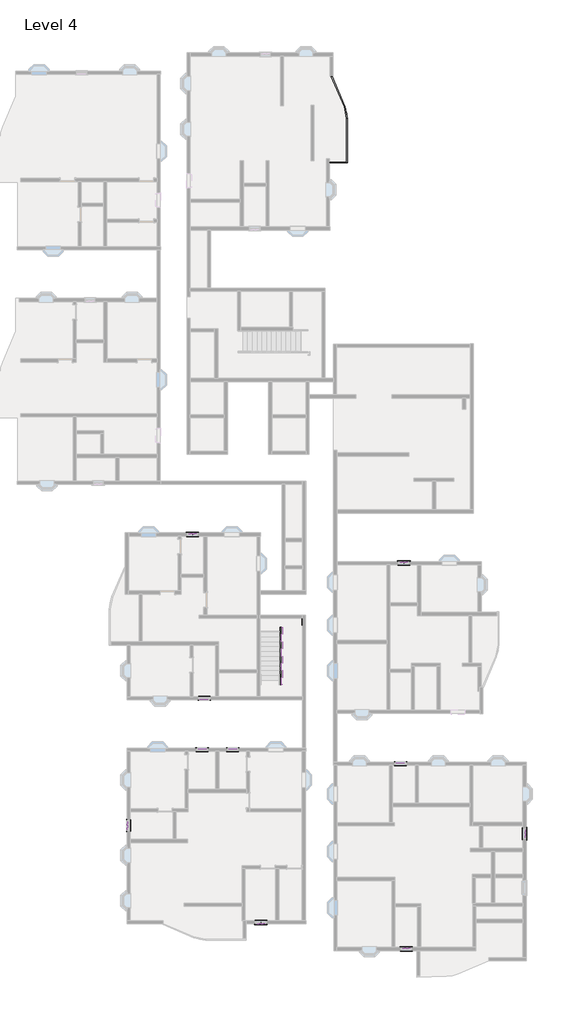
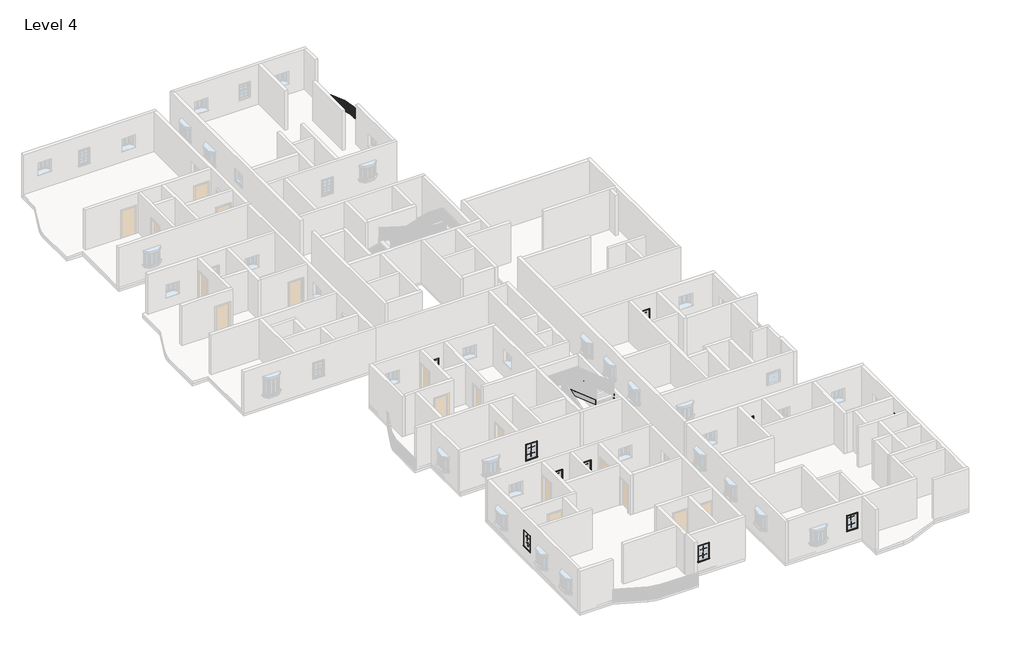
# One storey, part 13 of 14: 40 proxies, 6 members, 1 railing.
"""IFC4 building model written with IfcOpenShell, lengths in millimetres."""

from ifc_helpers import new_model, si_unit, frame, origin, place, context, project, spatial, polyline, circle_curve, outline, extrude, transform, mapped, element, save
from ifc_brep_helpers import plane_surface, cylinder_surface, revolved_surface, advanced_brep
from components import muntin_pattern_2x2_muntin_pattern_2x2_c35c595f, trim_window_exterior_flat_with_sill_e38017c9, trim_window_interior_flat_picture_frame_d728ed12

model = new_model("IFC4")

# Units and contexts
model_context = context("Model", 3, world=origin())
ifc_project = project(units=[si_unit("LENGTHUNIT", "METRE", prefix="MILLI")], contexts=[model_context])

# Site, building, storey
site = spatial("IfcSite", under=ifc_project)
building = spatial("IfcBuilding", under=site)
storey = spatial("IfcBuildingStorey", under=building, Name="Level 4", Elevation=9144.0)

# Proxies
placement = place(None, origin())
muntin_pattern_2x2_muntin_pattern_2x2_shape = muntin_pattern_2x2_muntin_pattern_2x2_c35c595f(model_context)
element("IfcBuildingElementProxy", 1, Name="Muntin Pattern_2x2 : Muntin Pattern_2x2", ObjectType="Muntin Pattern_2x2 : Muntin Pattern_2x2", at=placement, inside=storey, context=model_context, shape_type="MappedRepresentation", body=[
    mapped(muntin_pattern_2x2_muntin_pattern_2x2_shape, transform((-8150.287215, -357.5666506, 10614.025), x_axis=(1.0, 0.0, 0.0), y_axis=(0.0, 1.0, 0.0), z_axis=(0.0, 0.0, 1.0))),
])
element("IfcBuildingElementProxy", 2, Name="Muntin Pattern_2x2 : Muntin Pattern_2x2", ObjectType="Muntin Pattern_2x2 : Muntin Pattern_2x2", at=placement, inside=storey, context=model_context, shape_type="MappedRepresentation", body=[
    mapped(muntin_pattern_2x2_muntin_pattern_2x2_shape, transform((-8150.287215, -402.0166506, 10134.6), x_axis=(1.0, 0.0, 0.0), y_axis=(0.0, 1.0, 0.0), z_axis=(0.0, 0.0, 1.0))),
])
element("IfcBuildingElementProxy", 3, Name="Muntin Pattern_2x2 : Muntin Pattern_2x2", ObjectType="Muntin Pattern_2x2 : Muntin Pattern_2x2", at=placement, inside=storey, context=model_context, shape_type="MappedRepresentation", body=[
    mapped(muntin_pattern_2x2_muntin_pattern_2x2_shape, transform((-7397.812215, -10854.1166506, 10614.025), x_axis=(-1.0, 0.0, 0.0), y_axis=(0.0, -1.0, 0.0), z_axis=(0.0, 0.0, 1.0))),
])
element("IfcBuildingElementProxy", 4, Name="Muntin Pattern_2x2 : Muntin Pattern_2x2", ObjectType="Muntin Pattern_2x2 : Muntin Pattern_2x2", at=placement, inside=storey, context=model_context, shape_type="MappedRepresentation", body=[
    mapped(muntin_pattern_2x2_muntin_pattern_2x2_shape, transform((-7397.812215, -10809.6666506, 10134.6), x_axis=(-1.0, 0.0, 0.0), y_axis=(0.0, -1.0, 0.0), z_axis=(0.0, 0.0, 1.0))),
])
element("IfcBuildingElementProxy", 5, Name="Muntin Pattern_2x2 : Muntin Pattern_2x2", ObjectType="Muntin Pattern_2x2 : Muntin Pattern_2x2", at=placement, inside=storey, context=model_context, shape_type="MappedRepresentation", body=[
    mapped(muntin_pattern_2x2_muntin_pattern_2x2_shape, transform((-7540.687215, -13997.3666506, 10614.025), x_axis=(1.0, 0.0, 0.0), y_axis=(0.0, 1.0, 0.0), z_axis=(0.0, 0.0, 1.0))),
])
element("IfcBuildingElementProxy", 6, Name="Muntin Pattern_2x2 : Muntin Pattern_2x2", ObjectType="Muntin Pattern_2x2 : Muntin Pattern_2x2", at=placement, inside=storey, context=model_context, shape_type="MappedRepresentation", body=[
    mapped(muntin_pattern_2x2_muntin_pattern_2x2_shape, transform((-7540.687215, -14041.8166506, 10134.6), x_axis=(1.0, 0.0, 0.0), y_axis=(0.0, 1.0, 0.0), z_axis=(0.0, 0.0, 1.0))),
])
element("IfcBuildingElementProxy", 7, Name="Muntin Pattern_2x2 : Muntin Pattern_2x2", ObjectType="Muntin Pattern_2x2 : Muntin Pattern_2x2", at=placement, inside=storey, context=model_context, shape_type="MappedRepresentation", body=[
    mapped(muntin_pattern_2x2_muntin_pattern_2x2_shape, transform((-5597.587215, -13997.3666506, 10614.025), x_axis=(1.0, 0.0, 0.0), y_axis=(0.0, 1.0, 0.0), z_axis=(0.0, 0.0, 1.0))),
])
element("IfcBuildingElementProxy", 8, Name="Muntin Pattern_2x2 : Muntin Pattern_2x2", ObjectType="Muntin Pattern_2x2 : Muntin Pattern_2x2", at=placement, inside=storey, context=model_context, shape_type="MappedRepresentation", body=[
    mapped(muntin_pattern_2x2_muntin_pattern_2x2_shape, transform((-5597.587215, -14041.8166506, 10134.6), x_axis=(1.0, 0.0, 0.0), y_axis=(0.0, 1.0, 0.0), z_axis=(0.0, 0.0, 1.0))),
])
element("IfcBuildingElementProxy", 9, Name="Muntin Pattern_2x2 : Muntin Pattern_2x2", ObjectType="Muntin Pattern_2x2 : Muntin Pattern_2x2", at=placement, inside=storey, context=model_context, shape_type="MappedRepresentation", body=[
    mapped(muntin_pattern_2x2_muntin_pattern_2x2_shape, transform((-12255.562215, -18863.6994419, 10614.025), x_axis=(0.0, 1.0, 0.0), y_axis=(-1.0, 0.0, 0.0), z_axis=(0.0, 0.0, 1.0))),
])
element("IfcBuildingElementProxy", 10, Name="Muntin Pattern_2x2 : Muntin Pattern_2x2", ObjectType="Muntin Pattern_2x2 : Muntin Pattern_2x2", at=placement, inside=storey, context=model_context, shape_type="MappedRepresentation", body=[
    mapped(muntin_pattern_2x2_muntin_pattern_2x2_shape, transform((-12211.112215, -18863.6994419, 10134.6), x_axis=(0.0, 1.0, 0.0), y_axis=(-1.0, 0.0, 0.0), z_axis=(0.0, 0.0, 1.0))),
])
element("IfcBuildingElementProxy", 11, Name="Muntin Pattern_2x2 : Muntin Pattern_2x2", ObjectType="Muntin Pattern_2x2 : Muntin Pattern_2x2", at=placement, inside=storey, context=model_context, shape_type="MappedRepresentation", body=[
    mapped(muntin_pattern_2x2_muntin_pattern_2x2_shape, transform((-3806.2891351, -25065.4166506, 10614.025), x_axis=(-1.0, 0.0, 0.0), y_axis=(0.0, -1.0, 0.0), z_axis=(0.0, 0.0, 1.0))),
])
element("IfcBuildingElementProxy", 12, Name="Muntin Pattern_2x2 : Muntin Pattern_2x2", ObjectType="Muntin Pattern_2x2 : Muntin Pattern_2x2", at=placement, inside=storey, context=model_context, shape_type="MappedRepresentation", body=[
    mapped(muntin_pattern_2x2_muntin_pattern_2x2_shape, transform((-3806.2891351, -25020.9666506, 10134.6), x_axis=(-1.0, 0.0, 0.0), y_axis=(0.0, -1.0, 0.0), z_axis=(0.0, 0.0, 1.0))),
])
element("IfcBuildingElementProxy", 13, Name="Muntin Pattern_2x2 : Muntin Pattern_2x2", ObjectType="Muntin Pattern_2x2 : Muntin Pattern_2x2", at=placement, inside=storey, context=model_context, shape_type="MappedRepresentation", body=[
    mapped(muntin_pattern_2x2_muntin_pattern_2x2_shape, transform((5410.0380523, -26615.6292694, 10614.025), x_axis=(1.0, 0.0, 0.0), y_axis=(0.0, 1.0, 0.0), z_axis=(0.0, 0.0, 1.0))),
])
element("IfcBuildingElementProxy", 14, Name="Muntin Pattern_2x2 : Muntin Pattern_2x2", ObjectType="Muntin Pattern_2x2 : Muntin Pattern_2x2", at=placement, inside=storey, context=model_context, shape_type="MappedRepresentation", body=[
    mapped(muntin_pattern_2x2_muntin_pattern_2x2_shape, transform((5410.0380523, -26660.0792694, 10134.6), x_axis=(1.0, 0.0, 0.0), y_axis=(0.0, 1.0, 0.0), z_axis=(0.0, 0.0, 1.0))),
])
element("IfcBuildingElementProxy", 15, Name="Muntin Pattern_2x2 : Muntin Pattern_2x2", ObjectType="Muntin Pattern_2x2 : Muntin Pattern_2x2", at=placement, inside=storey, context=model_context, shape_type="MappedRepresentation", body=[
    mapped(muntin_pattern_2x2_muntin_pattern_2x2_shape, transform((12982.4130523, -19379.8042694, 10614.025), x_axis=(0.0, -1.0, 0.0), y_axis=(1.0, 0.0, 0.0), z_axis=(0.0, 0.0, 1.0))),
])
element("IfcBuildingElementProxy", 16, Name="Muntin Pattern_2x2 : Muntin Pattern_2x2", ObjectType="Muntin Pattern_2x2 : Muntin Pattern_2x2", at=placement, inside=storey, context=model_context, shape_type="MappedRepresentation", body=[
    mapped(muntin_pattern_2x2_muntin_pattern_2x2_shape, transform((12937.9630523, -19379.8042694, 10134.6), x_axis=(0.0, -1.0, 0.0), y_axis=(1.0, 0.0, 0.0), z_axis=(0.0, 0.0, 1.0))),
])
element("IfcBuildingElementProxy", 17, Name="Muntin Pattern_2x2 : Muntin Pattern_2x2", ObjectType="Muntin Pattern_2x2 : Muntin Pattern_2x2", at=placement, inside=storey, context=model_context, shape_type="MappedRepresentation", body=[
    mapped(muntin_pattern_2x2_muntin_pattern_2x2_shape, transform((5048.0880523, -14880.8292694, 10614.025), x_axis=(1.0, 0.0, 0.0), y_axis=(0.0, 1.0, 0.0), z_axis=(0.0, 0.0, 1.0))),
])
element("IfcBuildingElementProxy", 18, Name="Muntin Pattern_2x2 : Muntin Pattern_2x2", ObjectType="Muntin Pattern_2x2 : Muntin Pattern_2x2", at=placement, inside=storey, context=model_context, shape_type="MappedRepresentation", body=[
    mapped(muntin_pattern_2x2_muntin_pattern_2x2_shape, transform((5048.0880523, -14925.2792694, 10134.6), x_axis=(1.0, 0.0, 0.0), y_axis=(0.0, 1.0, 0.0), z_axis=(0.0, 0.0, 1.0))),
])
element("IfcBuildingElementProxy", 19, Name="Muntin Pattern_2x2 : Muntin Pattern_2x2", ObjectType="Muntin Pattern_2x2 : Muntin Pattern_2x2", at=placement, inside=storey, context=model_context, shape_type="MappedRepresentation", body=[
    mapped(muntin_pattern_2x2_muntin_pattern_2x2_shape, transform((5257.6380523, -2168.1292694, 10614.025), x_axis=(1.0, 0.0, 0.0), y_axis=(0.0, 1.0, 0.0), z_axis=(0.0, 0.0, 1.0))),
])
element("IfcBuildingElementProxy", 20, Name="Muntin Pattern_2x2 : Muntin Pattern_2x2", ObjectType="Muntin Pattern_2x2 : Muntin Pattern_2x2", at=placement, inside=storey, context=model_context, shape_type="MappedRepresentation", body=[
    mapped(muntin_pattern_2x2_muntin_pattern_2x2_shape, transform((5257.6380523, -2212.5792694, 10134.6), x_axis=(1.0, 0.0, 0.0), y_axis=(0.0, 1.0, 0.0), z_axis=(0.0, 0.0, 1.0))),
])
trim_window_exterior_flat_with_sill_shape = trim_window_exterior_flat_with_sill_e38017c9(model_context)
element("IfcBuildingElementProxy", 21, Name="Trim-Window-Exterior-Flat : with Sill", ObjectType="Trim-Window-Exterior-Flat : with Sill", at=placement, inside=storey, context=model_context, shape_type="MappedRepresentation", body=[
    mapped(trim_window_exterior_flat_with_sill_shape, transform((-8150.287215, -322.6416506, 11125.2), x_axis=(-1.0, 0.0, 0.0), y_axis=(0.0, 0.0, 1.0), z_axis=(0.0, 1.0, 0.0))),
])
element("IfcBuildingElementProxy", 22, Name="Trim-Window-Exterior-Flat : with Sill", ObjectType="Trim-Window-Exterior-Flat : with Sill", at=placement, inside=storey, context=model_context, shape_type="MappedRepresentation", body=[
    mapped(trim_window_exterior_flat_with_sill_shape, transform((-7397.812215, -10889.0416506, 11125.2), x_axis=(1.0, 0.0, 0.0), y_axis=(0.0, 0.0, 1.0), z_axis=(0.0, -1.0, 0.0))),
])
element("IfcBuildingElementProxy", 23, Name="Trim-Window-Exterior-Flat : with Sill", ObjectType="Trim-Window-Exterior-Flat : with Sill", at=placement, inside=storey, context=model_context, shape_type="MappedRepresentation", body=[
    mapped(trim_window_exterior_flat_with_sill_shape, transform((-7540.687215, -13962.4416506, 11125.2), x_axis=(-1.0, 0.0, 0.0), y_axis=(0.0, 0.0, 1.0), z_axis=(0.0, 1.0, 0.0))),
])
element("IfcBuildingElementProxy", 24, Name="Trim-Window-Exterior-Flat : with Sill", ObjectType="Trim-Window-Exterior-Flat : with Sill", at=placement, inside=storey, context=model_context, shape_type="MappedRepresentation", body=[
    mapped(trim_window_exterior_flat_with_sill_shape, transform((-5597.587215, -13962.4416506, 11125.2), x_axis=(-1.0, 0.0, 0.0), y_axis=(0.0, 0.0, 1.0), z_axis=(0.0, 1.0, 0.0))),
])
element("IfcBuildingElementProxy", 25, Name="Trim-Window-Exterior-Flat : with Sill", ObjectType="Trim-Window-Exterior-Flat : with Sill", at=placement, inside=storey, context=model_context, shape_type="MappedRepresentation", body=[
    mapped(trim_window_exterior_flat_with_sill_shape, transform((-12290.487215, -18863.6994419, 11125.2), x_axis=(0.0, -1.0, 0.0), y_axis=(0.0, 0.0, 1.0), z_axis=(-1.0, 0.0, 0.0))),
])
element("IfcBuildingElementProxy", 26, Name="Trim-Window-Exterior-Flat : with Sill", ObjectType="Trim-Window-Exterior-Flat : with Sill", at=placement, inside=storey, context=model_context, shape_type="MappedRepresentation", body=[
    mapped(trim_window_exterior_flat_with_sill_shape, transform((-3806.2891351, -25100.3416506, 11125.2), x_axis=(1.0, 0.0, 0.0), y_axis=(0.0, 0.0, 1.0), z_axis=(0.0, -1.0, 0.0))),
])
element("IfcBuildingElementProxy", 27, Name="Trim-Window-Exterior-Flat : with Sill", ObjectType="Trim-Window-Exterior-Flat : with Sill", at=placement, inside=storey, context=model_context, shape_type="MappedRepresentation", body=[
    mapped(trim_window_exterior_flat_with_sill_shape, transform((5410.0380523, -26580.7042694, 11125.2), x_axis=(-1.0, 0.0, 0.0), y_axis=(0.0, 0.0, 1.0), z_axis=(0.0, 1.0, 0.0))),
])
element("IfcBuildingElementProxy", 28, Name="Trim-Window-Exterior-Flat : with Sill", ObjectType="Trim-Window-Exterior-Flat : with Sill", at=placement, inside=storey, context=model_context, shape_type="MappedRepresentation", body=[
    mapped(trim_window_exterior_flat_with_sill_shape, transform((13017.3380523, -19379.8042694, 11125.2), x_axis=(0.0, 1.0, 0.0), y_axis=(0.0, 0.0, 1.0), z_axis=(1.0, 0.0, 0.0))),
])
element("IfcBuildingElementProxy", 29, Name="Trim-Window-Exterior-Flat : with Sill", ObjectType="Trim-Window-Exterior-Flat : with Sill", at=placement, inside=storey, context=model_context, shape_type="MappedRepresentation", body=[
    mapped(trim_window_exterior_flat_with_sill_shape, transform((5048.0880523, -14845.9042694, 11125.2), x_axis=(-1.0, 0.0, 0.0), y_axis=(0.0, 0.0, 1.0), z_axis=(0.0, 1.0, 0.0))),
])
element("IfcBuildingElementProxy", 30, Name="Trim-Window-Exterior-Flat : with Sill", ObjectType="Trim-Window-Exterior-Flat : with Sill", at=placement, inside=storey, context=model_context, shape_type="MappedRepresentation", body=[
    mapped(trim_window_exterior_flat_with_sill_shape, transform((5257.6380523, -2133.2042694, 11125.2), x_axis=(-1.0, 0.0, 0.0), y_axis=(0.0, 0.0, 1.0), z_axis=(0.0, 1.0, 0.0))),
])
trim_window_interior_flat_picture_frame_shape = trim_window_interior_flat_picture_frame_d728ed12(model_context)
element("IfcBuildingElementProxy", 31, Name="Trim-Window-Interior-Flat : Picture Frame", ObjectType="Trim-Window-Interior-Flat : Picture Frame", at=placement, inside=storey, context=model_context, shape_type="MappedRepresentation", body=[
    mapped(trim_window_interior_flat_picture_frame_shape, transform((-8150.287215, -525.8416506, 11125.2), x_axis=(1.0, 0.0, 0.0), y_axis=(0.0, 0.0, 1.0), z_axis=(0.0, -1.0, 0.0))),
])
element("IfcBuildingElementProxy", 32, Name="Trim-Window-Interior-Flat : Picture Frame", ObjectType="Trim-Window-Interior-Flat : Picture Frame", at=placement, inside=storey, context=model_context, shape_type="MappedRepresentation", body=[
    mapped(trim_window_interior_flat_picture_frame_shape, transform((-7397.812215, -10685.8416506, 11125.2), x_axis=(-1.0, 0.0, 0.0), y_axis=(0.0, 0.0, 1.0), z_axis=(0.0, 1.0, 0.0))),
])
element("IfcBuildingElementProxy", 33, Name="Trim-Window-Interior-Flat : Picture Frame", ObjectType="Trim-Window-Interior-Flat : Picture Frame", at=placement, inside=storey, context=model_context, shape_type="MappedRepresentation", body=[
    mapped(trim_window_interior_flat_picture_frame_shape, transform((-7540.687215, -14165.6416506, 11125.2), x_axis=(1.0, 0.0, 0.0), y_axis=(0.0, 0.0, 1.0), z_axis=(0.0, -1.0, 0.0))),
])
element("IfcBuildingElementProxy", 34, Name="Trim-Window-Interior-Flat : Picture Frame", ObjectType="Trim-Window-Interior-Flat : Picture Frame", at=placement, inside=storey, context=model_context, shape_type="MappedRepresentation", body=[
    mapped(trim_window_interior_flat_picture_frame_shape, transform((-5597.587215, -14165.6416506, 11125.2), x_axis=(1.0, 0.0, 0.0), y_axis=(0.0, 0.0, 1.0), z_axis=(0.0, -1.0, 0.0))),
])
element("IfcBuildingElementProxy", 35, Name="Trim-Window-Interior-Flat : Picture Frame", ObjectType="Trim-Window-Interior-Flat : Picture Frame", at=placement, inside=storey, context=model_context, shape_type="MappedRepresentation", body=[
    mapped(trim_window_interior_flat_picture_frame_shape, transform((-12087.287215, -18863.6994419, 11125.2), x_axis=(0.0, 1.0, 0.0), y_axis=(0.0, 0.0, 1.0), z_axis=(1.0, 0.0, 0.0))),
])
element("IfcBuildingElementProxy", 36, Name="Trim-Window-Interior-Flat : Picture Frame", ObjectType="Trim-Window-Interior-Flat : Picture Frame", at=placement, inside=storey, context=model_context, shape_type="MappedRepresentation", body=[
    mapped(trim_window_interior_flat_picture_frame_shape, transform((-3806.2891351, -24897.1416506, 11125.2), x_axis=(-1.0, 0.0, 0.0), y_axis=(0.0, 0.0, 1.0), z_axis=(0.0, 1.0, 0.0))),
])
element("IfcBuildingElementProxy", 37, Name="Trim-Window-Interior-Flat : Picture Frame", ObjectType="Trim-Window-Interior-Flat : Picture Frame", at=placement, inside=storey, context=model_context, shape_type="MappedRepresentation", body=[
    mapped(trim_window_interior_flat_picture_frame_shape, transform((5410.0380523, -26783.9042694, 11125.2), x_axis=(1.0, 0.0, 0.0), y_axis=(0.0, 0.0, 1.0), z_axis=(0.0, -1.0, 0.0))),
])
element("IfcBuildingElementProxy", 38, Name="Trim-Window-Interior-Flat : Picture Frame", ObjectType="Trim-Window-Interior-Flat : Picture Frame", at=placement, inside=storey, context=model_context, shape_type="MappedRepresentation", body=[
    mapped(trim_window_interior_flat_picture_frame_shape, transform((12814.1380523, -19379.8042694, 11125.2), x_axis=(0.0, -1.0, 0.0), y_axis=(0.0, 0.0, 1.0), z_axis=(-1.0, 0.0, 0.0))),
])
element("IfcBuildingElementProxy", 39, Name="Trim-Window-Interior-Flat : Picture Frame", ObjectType="Trim-Window-Interior-Flat : Picture Frame", at=placement, inside=storey, context=model_context, shape_type="MappedRepresentation", body=[
    mapped(trim_window_interior_flat_picture_frame_shape, transform((5048.0880523, -15049.1042694, 11125.2), x_axis=(1.0, 0.0, 0.0), y_axis=(0.0, 0.0, 1.0), z_axis=(0.0, -1.0, 0.0))),
])
element("IfcBuildingElementProxy", 40, Name="Trim-Window-Interior-Flat : Picture Frame", ObjectType="Trim-Window-Interior-Flat : Picture Frame", at=placement, inside=storey, context=model_context, shape_type="MappedRepresentation", body=[
    mapped(trim_window_interior_flat_picture_frame_shape, transform((5257.6380523, -2336.4042694, 11125.2), x_axis=(1.0, 0.0, 0.0), y_axis=(0.0, 0.0, 1.0), z_axis=(0.0, -1.0, 0.0))),
])

# Members
element("IfcMember", 41, ObjectType="Stringer - 2\" Width", at=placement, inside=storey, context=model_context, shape_type="SweptSolid", body=[
    extrude(outline(polyline([(-9955.5916506, 9144.0), (-9955.5916506, 9335.3592169), (-6325.8738327, 10591.8), (-5713.7916506, 10591.8), (-5713.7916506, 10481.1301656), (-9576.612129, 9144.0), (-9955.5916506, 9144.0)])), frame((-3908.487215, 0.0, 0.0), z_axis=(1.0, 0.0, 0.0), x_axis=(0.0, 1.0, 0.0)), (0.0, 0.0, 1.0), 50.8),
])
element("IfcMember", 42, ObjectType="Stringer - 2\" Width", at=placement, inside=storey, context=model_context, shape_type="SweptSolid", body=[
    extrude(outline(polyline([(-3908.487215, -5713.7916506), (-3908.487215, -5662.9916506), (-1190.687215, -5662.9916506), (-1190.687215, -5713.7916506), (-3908.487215, -5713.7916506)])), frame((0.0, 0.0, 10287.0), z_axis=(0.0, 0.0, 1.0), x_axis=(1.0, 0.0, 0.0)), (0.0, 0.0, 1.0), 304.8),
])
element("IfcMember", 43, ObjectType="Stringer - 2\" Width", at=placement, inside=storey, context=model_context, shape_type="SweptSolid", body=[
    extrude(outline(polyline([(-5662.9916506, 10491.5476784), (-5662.9916506, 10287.0), (-6003.8711722, 10287.0), (-9949.2416506, 11652.7051656), (-9949.2416506, 11975.2496015), (-5662.9916506, 10491.5476784)])), frame((-1190.687215, 0.0, 0.0), z_axis=(1.0, 0.0, 0.0), x_axis=(0.0, 1.0, 0.0)), (0.0, 0.0, 1.0), 50.8),
])
element("IfcMember", 44, ObjectType="Stringer - 2\" Width", at=placement, inside=storey, context=model_context, shape_type="SweptSolid", body=[
    extrude(outline(polyline([(-9955.5916506, 9144.0), (-9955.5916506, 9335.3592169), (-6342.4416506, 10586.0649861), (-6342.4416506, 10263.5205502), (-9576.612129, 9144.0), (-9955.5916506, 9144.0)])), frame((-2593.7381751, 0.0, 0.0), z_axis=(1.0, 0.0, 0.0), x_axis=(0.0, 1.0, 0.0)), (0.0, 0.0, 1.0), 50.8),
])
element("IfcMember", 45, ObjectType="Stringer - 2\" Width", at=placement, inside=storey, context=model_context, shape_type="SweptSolid", body=[
    extrude(outline(polyline([(-2593.7381751, -6342.4416506), (-2593.7381751, -6291.6416506), (-2492.1381751, -6291.6416506), (-2492.1381751, -6342.4416506), (-2593.7381751, -6342.4416506)])), frame((0.0, 0.0, 10287.0), z_axis=(0.0, 0.0, 1.0), x_axis=(1.0, 0.0, 0.0)), (0.0, 0.0, 1.0), 304.8),
])
element("IfcMember", 46, ObjectType="Stringer - 2\" Width", at=placement, inside=storey, context=model_context, shape_type="SweptSolid", body=[
    extrude(outline(polyline([(-6291.6416506, 10709.1572938), (-6291.6416506, 10386.6128579), (-9949.2416506, 11652.7051656), (-9949.2416506, 11975.2496015), (-6291.6416506, 10709.1572938)])), frame((-2492.1381751, 0.0, 0.0), z_axis=(1.0, 0.0, 0.0), x_axis=(0.0, 1.0, 0.0)), (0.0, 0.0, 1.0), 50.8),
])

# Railing
element("IfcRailing", 47, ObjectType="Handrail - Rectangular", at=placement, inside=storey, context=model_context, shape_type="SolidModel", body=[
    advanced_brep(
    [(549.8108649, 23180.4215905, 10058.4), (549.8108649, 23180.4215905, 10007.6), (549.8108649, 23129.6215905, 10007.6), (549.8108649, 23129.6215905, 10058.4), (1629.3108649, 23180.4215905, 10058.4), (1629.3108649, 23180.4215905, 10007.6), (1680.1108649, 23129.6215905, 10007.6), (1680.1108649, 23129.6215905, 10058.4), (1629.3108649, 25921.9580583, 10058.4), (1629.3108649, 25921.9580583, 10007.6), (1680.1108649, 25921.9580583, 10007.6), (1680.1108649, 25921.9580583, 10058.4), (1475.5051478, 26671.8537734, 10007.6), (1475.5051478, 26671.8537734, 10058.4), (1522.203662, 26691.8509925, 10007.6), (1522.203662, 26691.8509925, 10058.4), (640.7616078, 28621.188975, 10058.4), (687.460122, 28641.186194, 10058.4), (687.460122, 28641.186194, 10007.6), (640.7616078, 28621.188975, 10007.6)],
    [
        (0, 1),
        (1, 2),
        (2, 3),
        (3, 0),
        (0, 4),
        (4, 5),
        (5, 1),
        (5, 6),
        (6, 2),
        (6, 7),
        (7, 3),
        (7, 4),
        (4, 8),
        (8, 9),
        (9, 5),
        (9, 10),
        (10, 6),
        (10, 11),
        (11, 7),
        (11, 8),
        (12, 9, circle_curve(frame((-275.6891351, 25921.9580583, 10007.6), z_axis=(0.0, 0.0, -1.0), x_axis=(1.0, 0.0, 0.0)), 1905.0)),
        (8, 13, circle_curve(frame((-275.6891351, 25921.9580583, 10058.4), z_axis=(0.0, 0.0, 1.0), x_axis=(1.0, 0.0, 0.0)), 1905.0)),
        (13, 12),
        (14, 10, circle_curve(frame((-275.6891351, 25921.9580583, 10007.6), z_axis=(0.0, 0.0, -1.0), x_axis=(1.0, 0.0, 0.0)), 1955.8)),
        (12, 14),
        (15, 11, circle_curve(frame((-275.6891351, 25921.9580583, 10058.4), z_axis=(0.0, 0.0, -1.0), x_axis=(1.0, 0.0, 0.0)), 1955.8)),
        (14, 15),
        (15, 13),
        (16, 17),
        (17, 18),
        (18, 19),
        (19, 16),
        (13, 16),
        (19, 12),
        (18, 14),
        (17, 15),
    ],
    [
        plane_surface(frame((549.8108649, 23155.0215905, 10058.4), z_axis=(-1.0, 0.0, 0.0), x_axis=(0.0, 1.0, 0.0))),
        plane_surface(frame((549.8108649, 23180.4215905, 10058.4), z_axis=(0.0, 1.0, 0.0), x_axis=(1.0, 0.0, 0.0))),
        plane_surface(frame((549.8108649, 23180.4215905, 10007.6), z_axis=(0.0, 0.0, -1.0), x_axis=(1.0, 0.0, 0.0))),
        plane_surface(frame((549.8108649, 23129.6215905, 10007.6), z_axis=(0.0, -1.0, 0.0), x_axis=(1.0, 0.0, 0.0))),
        plane_surface(frame((549.8108649, 23129.6215905, 10058.4), z_axis=(0.0, 0.0, 1.0), x_axis=(1.0, 0.0, 0.0))),
        plane_surface(frame((1629.3108649, 23180.4215905, 10058.4), z_axis=(-1.0, 0.0, 0.0), x_axis=(0.0, 1.0, 0.0))),
        plane_surface(frame((1629.3108649, 23180.4215905, 10007.6), z_axis=(0.0, 0.0, -1.0), x_axis=(0.0, 1.0, 0.0))),
        plane_surface(frame((1680.1108649, 23129.6215905, 10007.6), z_axis=(1.0, 0.0, 0.0), x_axis=(0.0, 1.0, 0.0))),
        plane_surface(frame((1680.1108649, 23129.6215905, 10058.4), z_axis=(0.0, 0.0, 1.0), x_axis=(0.0, 1.0, 0.0))),
        revolved_surface(polyline([(1629.3108649, 25921.9580583, 10058.4), (1629.3108649, 25921.9580583, 10007.6)]), (-275.6891351, 25921.9580583, 10058.4), (0.0, 0.0, 1.0)),
        plane_surface(frame((-275.6891351, 25921.9580583, 10007.6), z_axis=(0.0, 0.0, -1.0), x_axis=(1.0, 0.0, 0.0))),
        cylinder_surface(frame((-275.6891351, 25921.9580583, 10058.4), z_axis=(0.0, 0.0, 1.0), x_axis=(1.0, 0.0, 0.0)), 1955.8),
        plane_surface(frame((-275.6891351, 25921.9580583, 10058.4), z_axis=(0.0, 0.0, 1.0), x_axis=(1.0, 0.0, 0.0))),
        plane_surface(frame((664.1108649, 28631.1875845, 10058.4), z_axis=(-0.39364604467361036, 0.91926209076238, 0.0), x_axis=(0.91926209076238, 0.39364604467361036, 0.0))),
        plane_surface(frame((1475.5051478, 26671.8537734, 10058.4), z_axis=(-0.91926209076238, -0.3936460446736102, 0.0), x_axis=(-0.3936460446736102, 0.91926209076238, 0.0))),
        plane_surface(frame((1475.5051478, 26671.8537734, 10007.6), z_axis=(0.0, 0.0, -1.0), x_axis=(-0.3936460446736102, 0.91926209076238, 0.0))),
        plane_surface(frame((1522.203662, 26691.8509925, 10007.6), z_axis=(0.91926209076238, 0.3936460446736102, 0.0), x_axis=(-0.3936460446736102, 0.91926209076238, 0.0))),
        plane_surface(frame((1522.203662, 26691.8509925, 10058.4), z_axis=(0.0, 0.0, 1.0), x_axis=(-0.3936460446736102, 0.91926209076238, 0.0))),
    ],
    [
        (0, [[1, 2, 3, 4]]),
        (1, [[-1, 5, 6, 7]]),
        (2, [[-2, -7, 8, 9]]),
        (3, [[-3, -9, 10, 11]]),
        (4, [[-4, -11, 12, -5]]),
        (5, [[-6, 13, 14, 15]]),
        (6, [[-8, -15, 16, 17]]),
        (7, [[-10, -17, 18, 19]]),
        (8, [[-12, -19, 20, -13]]),
        (9, [[21, -14, 22, 23]]),
        (10, [[24, -16, -21, 25]]),
        (11, [[26, -18, -24, 27]]),
        (12, [[-22, -20, -26, 28]]),
        (13, [[29, 30, 31, 32]]),
        (14, [[-23, 33, -32, 34]]),
        (15, [[-25, -34, -31, 35]]),
        (16, [[-27, -35, -30, 36]]),
        (17, [[-28, -36, -29, -33]]),
    ],
),
    extrude(outline(polyline([(711.4710921, 28544.7864585), (693.9591493, 28537.2875014), (686.4601921, 28554.7994442), (703.9721349, 28562.2984014), (711.4710921, 28544.7864585)])), frame((0.0, 0.0, 9144.0), z_axis=(0.0, 0.0, 1.0), x_axis=(1.0, 0.0, 0.0)), (0.0, 0.0, 1.0), 863.6),
    extrude(outline(polyline([(751.4655302, 28451.3894301), (733.9535874, 28443.890473), (726.4546303, 28461.4024158), (743.9665731, 28468.9013729), (751.4655302, 28451.3894301)])), frame((0.0, 0.0, 9144.0), z_axis=(0.0, 0.0, 1.0), x_axis=(1.0, 0.0, 0.0)), (0.0, 0.0, 1.0), 863.6),
    extrude(outline(polyline([(791.4599684, 28357.9924017), (773.9480255, 28350.4934445), (766.4490684, 28368.0053874), (783.9610112, 28375.5043445), (791.4599684, 28357.9924017)])), frame((0.0, 0.0, 9144.0), z_axis=(0.0, 0.0, 1.0), x_axis=(1.0, 0.0, 0.0)), (0.0, 0.0, 1.0), 863.6),
    extrude(outline(polyline([(831.4544065, 28264.5953733), (813.9424637, 28257.0964161), (806.4435065, 28274.608359), (823.9554494, 28282.1073161), (831.4544065, 28264.5953733)])), frame((0.0, 0.0, 9144.0), z_axis=(0.0, 0.0, 1.0), x_axis=(1.0, 0.0, 0.0)), (0.0, 0.0, 1.0), 863.6),
    extrude(outline(polyline([(871.4488446, 28171.1983449), (853.9369018, 28163.6993877), (846.4379447, 28181.2113305), (863.9498875, 28188.7102877), (871.4488446, 28171.1983449)])), frame((0.0, 0.0, 9144.0), z_axis=(0.0, 0.0, 1.0), x_axis=(1.0, 0.0, 0.0)), (0.0, 0.0, 1.0), 863.6),
    extrude(outline(polyline([(911.4432828, 28077.8013164), (893.93134, 28070.3023593), (886.4323828, 28087.8143021), (903.9443256, 28095.3132593), (911.4432828, 28077.8013164)])), frame((0.0, 0.0, 9144.0), z_axis=(0.0, 0.0, 1.0), x_axis=(1.0, 0.0, 0.0)), (0.0, 0.0, 1.0), 863.6),
    extrude(outline(polyline([(951.4377209, 27984.404288), (933.9257781, 27976.9053309), (926.4268209, 27994.4172737), (943.9387638, 28001.9162308), (951.4377209, 27984.404288)])), frame((0.0, 0.0, 9144.0), z_axis=(0.0, 0.0, 1.0), x_axis=(1.0, 0.0, 0.0)), (0.0, 0.0, 1.0), 863.6),
    extrude(outline(polyline([(991.4321591, 27891.0072596), (973.9202162, 27883.5083024), (966.4212591, 27901.0202453), (983.9332019, 27908.5192024), (991.4321591, 27891.0072596)])), frame((0.0, 0.0, 9144.0), z_axis=(0.0, 0.0, 1.0), x_axis=(1.0, 0.0, 0.0)), (0.0, 0.0, 1.0), 863.6),
    extrude(outline(polyline([(1031.4265972, 27797.6102312), (1013.9146544, 27790.111274), (1006.4156972, 27807.6232168), (1023.9276401, 27815.122174), (1031.4265972, 27797.6102312)])), frame((0.0, 0.0, 9144.0), z_axis=(0.0, 0.0, 1.0), x_axis=(1.0, 0.0, 0.0)), (0.0, 0.0, 1.0), 863.6),
    extrude(outline(polyline([(1071.4210353, 27704.2132027), (1053.9090925, 27696.7142456), (1046.4101354, 27714.2261884), (1063.9220782, 27721.7251456), (1071.4210353, 27704.2132027)])), frame((0.0, 0.0, 9144.0), z_axis=(0.0, 0.0, 1.0), x_axis=(1.0, 0.0, 0.0)), (0.0, 0.0, 1.0), 863.6),
    extrude(outline(polyline([(1111.4154735, 27610.8161743), (1093.9035307, 27603.3172172), (1086.4045735, 27620.82916), (1103.9165163, 27628.3281172), (1111.4154735, 27610.8161743)])), frame((0.0, 0.0, 9144.0), z_axis=(0.0, 0.0, 1.0), x_axis=(1.0, 0.0, 0.0)), (0.0, 0.0, 1.0), 863.6),
    extrude(outline(polyline([(1151.4099116, 27517.4191459), (1133.8979688, 27509.9201888), (1126.3990116, 27527.4321316), (1143.9109545, 27534.9310887), (1151.4099116, 27517.4191459)])), frame((0.0, 0.0, 9144.0), z_axis=(0.0, 0.0, 1.0), x_axis=(1.0, 0.0, 0.0)), (0.0, 0.0, 1.0), 863.6),
    extrude(outline(polyline([(1191.4043498, 27424.0221175), (1173.8924069, 27416.5231603), (1166.3934498, 27434.0351032), (1183.9053926, 27441.5340603), (1191.4043498, 27424.0221175)])), frame((0.0, 0.0, 9144.0), z_axis=(0.0, 0.0, 1.0), x_axis=(1.0, 0.0, 0.0)), (0.0, 0.0, 1.0), 863.6),
    extrude(outline(polyline([(1231.3987879, 27330.6250891), (1213.8868451, 27323.1261319), (1206.3878879, 27340.6380747), (1223.8998307, 27348.1370319), (1231.3987879, 27330.6250891)])), frame((0.0, 0.0, 9144.0), z_axis=(0.0, 0.0, 1.0), x_axis=(1.0, 0.0, 0.0)), (0.0, 0.0, 1.0), 863.6),
    extrude(outline(polyline([(1271.393226, 27237.2280606), (1253.8812832, 27229.7291035), (1246.3823261, 27247.2410463), (1263.8942689, 27254.7400035), (1271.393226, 27237.2280606)])), frame((0.0, 0.0, 9144.0), z_axis=(0.0, 0.0, 1.0), x_axis=(1.0, 0.0, 0.0)), (0.0, 0.0, 1.0), 863.6),
    extrude(outline(polyline([(1311.3876642, 27143.8310322), (1293.8757213, 27136.3320751), (1286.3767642, 27153.8440179), (1303.888707, 27161.342975), (1311.3876642, 27143.8310322)])), frame((0.0, 0.0, 9144.0), z_axis=(0.0, 0.0, 1.0), x_axis=(1.0, 0.0, 0.0)), (0.0, 0.0, 1.0), 863.6),
    extrude(outline(polyline([(1351.3821023, 27050.4340038), (1333.8701595, 27042.9350466), (1326.3712023, 27060.4469895), (1343.8831452, 27067.9459466), (1351.3821023, 27050.4340038)])), frame((0.0, 0.0, 9144.0), z_axis=(0.0, 0.0, 1.0), x_axis=(1.0, 0.0, 0.0)), (0.0, 0.0, 1.0), 863.6),
    extrude(outline(polyline([(1391.3765405, 26957.0369754), (1373.8645976, 26949.5380182), (1366.3656405, 26967.0499611), (1383.8775833, 26974.5489182), (1391.3765405, 26957.0369754)])), frame((0.0, 0.0, 9144.0), z_axis=(0.0, 0.0, 1.0), x_axis=(1.0, 0.0, 0.0)), (0.0, 0.0, 1.0), 863.6),
    extrude(outline(polyline([(1431.3709786, 26863.639947), (1413.8590358, 26856.1409898), (1406.3600786, 26873.6529326), (1423.8720214, 26881.1518898), (1431.3709786, 26863.639947)])), frame((0.0, 0.0, 9144.0), z_axis=(0.0, 0.0, 1.0), x_axis=(1.0, 0.0, 0.0)), (0.0, 0.0, 1.0), 863.6),
    extrude(outline(polyline([(1471.3654167, 26770.2429185), (1453.8534739, 26762.7439614), (1446.3545168, 26780.2559042), (1463.8664596, 26787.7548614), (1471.3654167, 26770.2429185)])), frame((0.0, 0.0, 9144.0), z_axis=(0.0, 0.0, 1.0), x_axis=(1.0, 0.0, 0.0)), (0.0, 0.0, 1.0), 863.6),
    extrude(outline(polyline([(1537.4917391, 26611.722401), (1519.7200483, 26604.8616791), (1512.8593263, 26622.6333699), (1530.6310171, 26629.4940918), (1537.4917391, 26611.722401)])), frame((0.0, 0.0, 9144.0), z_axis=(0.0, 0.0, 1.0), x_axis=(1.0, 0.0, 0.0)), (0.0, 0.0, 1.0), 863.6),
    extrude(outline(polyline([(1571.2676162, 26515.3807493), (1553.1596103, 26509.4644479), (1547.2433088, 26527.5724538), (1565.3513147, 26533.4887552), (1571.2676162, 26515.3807493)])), frame((0.0, 0.0, 9144.0), z_axis=(0.0, 0.0, 1.0), x_axis=(1.0, 0.0, 0.0)), (0.0, 0.0, 1.0), 863.6),
    extrude(outline(polyline([(1599.9284504, 26417.3956468), (1581.5342785, 26412.4401508), (1576.5787825, 26430.8343227), (1594.9729544, 26435.7898187), (1599.9284504, 26417.3956468)])), frame((0.0, 0.0, 9144.0), z_axis=(0.0, 0.0, 1.0), x_axis=(1.0, 0.0, 0.0)), (0.0, 0.0, 1.0), 863.6),
    extrude(outline(polyline([(1623.3948673, 26318.0384578), (1604.7654711, 26314.0574912), (1600.7845045, 26332.6868874), (1619.4139008, 26336.667854), (1623.3948673, 26318.0384578)])), frame((0.0, 0.0, 9144.0), z_axis=(0.0, 0.0, 1.0), x_axis=(1.0, 0.0, 0.0)), (0.0, 0.0, 1.0), 863.6),
    extrude(outline(polyline([(1641.601878, 26217.5843464), (1622.7888504, 26214.5889343), (1619.7934383, 26233.4019618), (1638.6064659, 26236.3973739), (1641.601878, 26217.5843464)])), frame((0.0, 0.0, 9144.0), z_axis=(0.0, 0.0, 1.0), x_axis=(1.0, 0.0, 0.0)), (0.0, 0.0, 1.0), 863.6),
    extrude(outline(polyline([(1654.4990591, 26116.3115146), (1635.5545019, 26114.3099526), (1633.5529398, 26133.2545098), (1652.4974971, 26135.2560719), (1654.4990591, 26116.3115146)])), frame((0.0, 0.0, 9144.0), z_axis=(0.0, 0.0, 1.0), x_axis=(1.0, 0.0, 0.0)), (0.0, 0.0, 1.0), 863.6),
    extrude(outline(polyline([(1662.0506927, 26014.5004319), (1643.0270716, 26013.4982632), (1642.0249029, 26032.5218842), (1661.048524, 26033.524053), (1662.0506927, 26014.5004319)])), frame((0.0, 0.0, 9144.0), z_axis=(0.0, 0.0, 1.0), x_axis=(1.0, 0.0, 0.0)), (0.0, 0.0, 1.0), 863.6),
    extrude(outline(polyline([(1664.2358649, 25888.6965905), (1645.1858649, 25888.6965905), (1645.1858649, 25907.7465905), (1664.2358649, 25907.7465905), (1664.2358649, 25888.6965905)])), frame((0.0, 0.0, 9144.0), z_axis=(0.0, 0.0, 1.0), x_axis=(1.0, 0.0, 0.0)), (0.0, 0.0, 1.0), 863.6),
    extrude(outline(polyline([(1664.2358649, 25787.0965905), (1645.1858649, 25787.0965905), (1645.1858649, 25806.1465905), (1664.2358649, 25806.1465905), (1664.2358649, 25787.0965905)])), frame((0.0, 0.0, 9144.0), z_axis=(0.0, 0.0, 1.0), x_axis=(1.0, 0.0, 0.0)), (0.0, 0.0, 1.0), 863.6),
    extrude(outline(polyline([(1664.2358649, 25685.4965905), (1645.1858649, 25685.4965905), (1645.1858649, 25704.5465905), (1664.2358649, 25704.5465905), (1664.2358649, 25685.4965905)])), frame((0.0, 0.0, 9144.0), z_axis=(0.0, 0.0, 1.0), x_axis=(1.0, 0.0, 0.0)), (0.0, 0.0, 1.0), 863.6),
    extrude(outline(polyline([(1664.2358649, 25583.8965905), (1645.1858649, 25583.8965905), (1645.1858649, 25602.9465905), (1664.2358649, 25602.9465905), (1664.2358649, 25583.8965905)])), frame((0.0, 0.0, 9144.0), z_axis=(0.0, 0.0, 1.0), x_axis=(1.0, 0.0, 0.0)), (0.0, 0.0, 1.0), 863.6),
    extrude(outline(polyline([(1664.2358649, 25482.2965905), (1645.1858649, 25482.2965905), (1645.1858649, 25501.3465905), (1664.2358649, 25501.3465905), (1664.2358649, 25482.2965905)])), frame((0.0, 0.0, 9144.0), z_axis=(0.0, 0.0, 1.0), x_axis=(1.0, 0.0, 0.0)), (0.0, 0.0, 1.0), 863.6),
    extrude(outline(polyline([(1664.2358649, 25380.6965905), (1645.1858649, 25380.6965905), (1645.1858649, 25399.7465905), (1664.2358649, 25399.7465905), (1664.2358649, 25380.6965905)])), frame((0.0, 0.0, 9144.0), z_axis=(0.0, 0.0, 1.0), x_axis=(1.0, 0.0, 0.0)), (0.0, 0.0, 1.0), 863.6),
    extrude(outline(polyline([(1664.2358649, 25279.0965905), (1645.1858649, 25279.0965905), (1645.1858649, 25298.1465905), (1664.2358649, 25298.1465905), (1664.2358649, 25279.0965905)])), frame((0.0, 0.0, 9144.0), z_axis=(0.0, 0.0, 1.0), x_axis=(1.0, 0.0, 0.0)), (0.0, 0.0, 1.0), 863.6),
    extrude(outline(polyline([(1664.2358649, 25177.4965905), (1645.1858649, 25177.4965905), (1645.1858649, 25196.5465905), (1664.2358649, 25196.5465905), (1664.2358649, 25177.4965905)])), frame((0.0, 0.0, 9144.0), z_axis=(0.0, 0.0, 1.0), x_axis=(1.0, 0.0, 0.0)), (0.0, 0.0, 1.0), 863.6),
    extrude(outline(polyline([(1664.2358649, 25075.8965905), (1645.1858649, 25075.8965905), (1645.1858649, 25094.9465905), (1664.2358649, 25094.9465905), (1664.2358649, 25075.8965905)])), frame((0.0, 0.0, 9144.0), z_axis=(0.0, 0.0, 1.0), x_axis=(1.0, 0.0, 0.0)), (0.0, 0.0, 1.0), 863.6),
    extrude(outline(polyline([(1664.2358649, 24974.2965905), (1645.1858649, 24974.2965905), (1645.1858649, 24993.3465905), (1664.2358649, 24993.3465905), (1664.2358649, 24974.2965905)])), frame((0.0, 0.0, 9144.0), z_axis=(0.0, 0.0, 1.0), x_axis=(1.0, 0.0, 0.0)), (0.0, 0.0, 1.0), 863.6),
    extrude(outline(polyline([(1664.2358649, 24872.6965905), (1645.1858649, 24872.6965905), (1645.1858649, 24891.7465905), (1664.2358649, 24891.7465905), (1664.2358649, 24872.6965905)])), frame((0.0, 0.0, 9144.0), z_axis=(0.0, 0.0, 1.0), x_axis=(1.0, 0.0, 0.0)), (0.0, 0.0, 1.0), 863.6),
    extrude(outline(polyline([(1664.2358649, 24771.0965905), (1645.1858649, 24771.0965905), (1645.1858649, 24790.1465905), (1664.2358649, 24790.1465905), (1664.2358649, 24771.0965905)])), frame((0.0, 0.0, 9144.0), z_axis=(0.0, 0.0, 1.0), x_axis=(1.0, 0.0, 0.0)), (0.0, 0.0, 1.0), 863.6),
    extrude(outline(polyline([(1664.2358649, 24669.4965905), (1645.1858649, 24669.4965905), (1645.1858649, 24688.5465905), (1664.2358649, 24688.5465905), (1664.2358649, 24669.4965905)])), frame((0.0, 0.0, 9144.0), z_axis=(0.0, 0.0, 1.0), x_axis=(1.0, 0.0, 0.0)), (0.0, 0.0, 1.0), 863.6),
    extrude(outline(polyline([(1664.2358649, 24567.8965905), (1645.1858649, 24567.8965905), (1645.1858649, 24586.9465905), (1664.2358649, 24586.9465905), (1664.2358649, 24567.8965905)])), frame((0.0, 0.0, 9144.0), z_axis=(0.0, 0.0, 1.0), x_axis=(1.0, 0.0, 0.0)), (0.0, 0.0, 1.0), 863.6),
    extrude(outline(polyline([(1664.2358649, 24466.2965905), (1645.1858649, 24466.2965905), (1645.1858649, 24485.3465905), (1664.2358649, 24485.3465905), (1664.2358649, 24466.2965905)])), frame((0.0, 0.0, 9144.0), z_axis=(0.0, 0.0, 1.0), x_axis=(1.0, 0.0, 0.0)), (0.0, 0.0, 1.0), 863.6),
    extrude(outline(polyline([(1664.2358649, 24364.6965905), (1645.1858649, 24364.6965905), (1645.1858649, 24383.7465905), (1664.2358649, 24383.7465905), (1664.2358649, 24364.6965905)])), frame((0.0, 0.0, 9144.0), z_axis=(0.0, 0.0, 1.0), x_axis=(1.0, 0.0, 0.0)), (0.0, 0.0, 1.0), 863.6),
    extrude(outline(polyline([(1664.2358649, 24263.0965905), (1645.1858649, 24263.0965905), (1645.1858649, 24282.1465905), (1664.2358649, 24282.1465905), (1664.2358649, 24263.0965905)])), frame((0.0, 0.0, 9144.0), z_axis=(0.0, 0.0, 1.0), x_axis=(1.0, 0.0, 0.0)), (0.0, 0.0, 1.0), 863.6),
    extrude(outline(polyline([(1664.2358649, 24161.4965905), (1645.1858649, 24161.4965905), (1645.1858649, 24180.5465905), (1664.2358649, 24180.5465905), (1664.2358649, 24161.4965905)])), frame((0.0, 0.0, 9144.0), z_axis=(0.0, 0.0, 1.0), x_axis=(1.0, 0.0, 0.0)), (0.0, 0.0, 1.0), 863.6),
    extrude(outline(polyline([(1664.2358649, 24059.8965905), (1645.1858649, 24059.8965905), (1645.1858649, 24078.9465905), (1664.2358649, 24078.9465905), (1664.2358649, 24059.8965905)])), frame((0.0, 0.0, 9144.0), z_axis=(0.0, 0.0, 1.0), x_axis=(1.0, 0.0, 0.0)), (0.0, 0.0, 1.0), 863.6),
    extrude(outline(polyline([(1664.2358649, 23958.2965905), (1645.1858649, 23958.2965905), (1645.1858649, 23977.3465905), (1664.2358649, 23977.3465905), (1664.2358649, 23958.2965905)])), frame((0.0, 0.0, 9144.0), z_axis=(0.0, 0.0, 1.0), x_axis=(1.0, 0.0, 0.0)), (0.0, 0.0, 1.0), 863.6),
    extrude(outline(polyline([(1664.2358649, 23856.6965905), (1645.1858649, 23856.6965905), (1645.1858649, 23875.7465905), (1664.2358649, 23875.7465905), (1664.2358649, 23856.6965905)])), frame((0.0, 0.0, 9144.0), z_axis=(0.0, 0.0, 1.0), x_axis=(1.0, 0.0, 0.0)), (0.0, 0.0, 1.0), 863.6),
    extrude(outline(polyline([(1664.2358649, 23755.0965905), (1645.1858649, 23755.0965905), (1645.1858649, 23774.1465905), (1664.2358649, 23774.1465905), (1664.2358649, 23755.0965905)])), frame((0.0, 0.0, 9144.0), z_axis=(0.0, 0.0, 1.0), x_axis=(1.0, 0.0, 0.0)), (0.0, 0.0, 1.0), 863.6),
    extrude(outline(polyline([(1664.2358649, 23653.4965905), (1645.1858649, 23653.4965905), (1645.1858649, 23672.5465905), (1664.2358649, 23672.5465905), (1664.2358649, 23653.4965905)])), frame((0.0, 0.0, 9144.0), z_axis=(0.0, 0.0, 1.0), x_axis=(1.0, 0.0, 0.0)), (0.0, 0.0, 1.0), 863.6),
    extrude(outline(polyline([(1664.2358649, 23551.8965905), (1645.1858649, 23551.8965905), (1645.1858649, 23570.9465905), (1664.2358649, 23570.9465905), (1664.2358649, 23551.8965905)])), frame((0.0, 0.0, 9144.0), z_axis=(0.0, 0.0, 1.0), x_axis=(1.0, 0.0, 0.0)), (0.0, 0.0, 1.0), 863.6),
    extrude(outline(polyline([(1664.2358649, 23450.2965905), (1645.1858649, 23450.2965905), (1645.1858649, 23469.3465905), (1664.2358649, 23469.3465905), (1664.2358649, 23450.2965905)])), frame((0.0, 0.0, 9144.0), z_axis=(0.0, 0.0, 1.0), x_axis=(1.0, 0.0, 0.0)), (0.0, 0.0, 1.0), 863.6),
    extrude(outline(polyline([(1664.2358649, 23348.6965905), (1645.1858649, 23348.6965905), (1645.1858649, 23367.7465905), (1664.2358649, 23367.7465905), (1664.2358649, 23348.6965905)])), frame((0.0, 0.0, 9144.0), z_axis=(0.0, 0.0, 1.0), x_axis=(1.0, 0.0, 0.0)), (0.0, 0.0, 1.0), 863.6),
    extrude(outline(polyline([(1664.2358649, 23247.0965905), (1645.1858649, 23247.0965905), (1645.1858649, 23266.1465905), (1664.2358649, 23266.1465905), (1664.2358649, 23247.0965905)])), frame((0.0, 0.0, 9144.0), z_axis=(0.0, 0.0, 1.0), x_axis=(1.0, 0.0, 0.0)), (0.0, 0.0, 1.0), 863.6),
    extrude(outline(polyline([(1556.2858649, 23145.4965905), (1556.2858649, 23164.5465905), (1575.3358649, 23164.5465905), (1575.3358649, 23145.4965905), (1556.2858649, 23145.4965905)])), frame((0.0, 0.0, 9144.0), z_axis=(0.0, 0.0, 1.0), x_axis=(1.0, 0.0, 0.0)), (0.0, 0.0, 1.0), 863.6),
    extrude(outline(polyline([(1454.6858649, 23145.4965905), (1454.6858649, 23164.5465905), (1473.7358649, 23164.5465905), (1473.7358649, 23145.4965905), (1454.6858649, 23145.4965905)])), frame((0.0, 0.0, 9144.0), z_axis=(0.0, 0.0, 1.0), x_axis=(1.0, 0.0, 0.0)), (0.0, 0.0, 1.0), 863.6),
    extrude(outline(polyline([(1353.0858649, 23145.4965905), (1353.0858649, 23164.5465905), (1372.1358649, 23164.5465905), (1372.1358649, 23145.4965905), (1353.0858649, 23145.4965905)])), frame((0.0, 0.0, 9144.0), z_axis=(0.0, 0.0, 1.0), x_axis=(1.0, 0.0, 0.0)), (0.0, 0.0, 1.0), 863.6),
    extrude(outline(polyline([(1251.4858649, 23145.4965905), (1251.4858649, 23164.5465905), (1270.5358649, 23164.5465905), (1270.5358649, 23145.4965905), (1251.4858649, 23145.4965905)])), frame((0.0, 0.0, 9144.0), z_axis=(0.0, 0.0, 1.0), x_axis=(1.0, 0.0, 0.0)), (0.0, 0.0, 1.0), 863.6),
    extrude(outline(polyline([(1149.8858649, 23145.4965905), (1149.8858649, 23164.5465905), (1168.9358649, 23164.5465905), (1168.9358649, 23145.4965905), (1149.8858649, 23145.4965905)])), frame((0.0, 0.0, 9144.0), z_axis=(0.0, 0.0, 1.0), x_axis=(1.0, 0.0, 0.0)), (0.0, 0.0, 1.0), 863.6),
    extrude(outline(polyline([(1048.2858649, 23145.4965905), (1048.2858649, 23164.5465905), (1067.3358649, 23164.5465905), (1067.3358649, 23145.4965905), (1048.2858649, 23145.4965905)])), frame((0.0, 0.0, 9144.0), z_axis=(0.0, 0.0, 1.0), x_axis=(1.0, 0.0, 0.0)), (0.0, 0.0, 1.0), 863.6),
    extrude(outline(polyline([(946.6858649, 23145.4965905), (946.6858649, 23164.5465905), (965.7358649, 23164.5465905), (965.7358649, 23145.4965905), (946.6858649, 23145.4965905)])), frame((0.0, 0.0, 9144.0), z_axis=(0.0, 0.0, 1.0), x_axis=(1.0, 0.0, 0.0)), (0.0, 0.0, 1.0), 863.6),
    extrude(outline(polyline([(845.0858649, 23145.4965905), (845.0858649, 23164.5465905), (864.1358649, 23164.5465905), (864.1358649, 23145.4965905), (845.0858649, 23145.4965905)])), frame((0.0, 0.0, 9144.0), z_axis=(0.0, 0.0, 1.0), x_axis=(1.0, 0.0, 0.0)), (0.0, 0.0, 1.0), 863.6),
    extrude(outline(polyline([(743.4858649, 23145.4965905), (743.4858649, 23164.5465905), (762.5358649, 23164.5465905), (762.5358649, 23145.4965905), (743.4858649, 23145.4965905)])), frame((0.0, 0.0, 9144.0), z_axis=(0.0, 0.0, 1.0), x_axis=(1.0, 0.0, 0.0)), (0.0, 0.0, 1.0), 863.6),
    extrude(outline(polyline([(641.8858649, 23145.4965905), (641.8858649, 23164.5465905), (660.9358649, 23164.5465905), (660.9358649, 23145.4965905), (641.8858649, 23145.4965905)])), frame((0.0, 0.0, 9144.0), z_axis=(0.0, 0.0, 1.0), x_axis=(1.0, 0.0, 0.0)), (0.0, 0.0, 1.0), 863.6),
    extrude(outline(polyline([(1511.3598549, 26676.8458901), (1493.847912, 26669.346933), (1486.3489549, 26686.8588758), (1503.8608977, 26694.3578329), (1511.3598549, 26676.8458901)])), frame((0.0, 0.0, 9144.0), z_axis=(0.0, 0.0, 1.0), x_axis=(1.0, 0.0, 0.0)), (0.0, 0.0, 1.0), 863.6),
    extrude(outline(polyline([(1664.2358649, 25912.4330583), (1645.1858649, 25912.4330583), (1645.1858649, 25931.4830583), (1664.2358649, 25931.4830583), (1664.2358649, 25912.4330583)])), frame((0.0, 0.0, 9144.0), z_axis=(0.0, 0.0, 1.0), x_axis=(1.0, 0.0, 0.0)), (0.0, 0.0, 1.0), 863.6),
    extrude(outline(polyline([(1645.1858649, 23145.4965905), (1645.1858649, 23164.5465905), (1664.2358649, 23164.5465905), (1664.2358649, 23145.4965905), (1645.1858649, 23145.4965905)])), frame((0.0, 0.0, 9144.0), z_axis=(0.0, 0.0, 1.0), x_axis=(1.0, 0.0, 0.0)), (0.0, 0.0, 1.0), 863.6),
    extrude(outline(polyline([(680.3657934, 28617.4251203), (662.8538506, 28609.9261631), (655.3548935, 28627.4381059), (672.8668363, 28634.9370631), (680.3657934, 28617.4251203)])), frame((0.0, 0.0, 9144.0), z_axis=(0.0, 0.0, 1.0), x_axis=(1.0, 0.0, 0.0)), (0.0, 0.0, 1.0), 863.6),
    extrude(outline(polyline([(549.8108649, 23145.4965905), (549.8108649, 23164.5465905), (568.8608649, 23164.5465905), (568.8608649, 23145.4965905), (549.8108649, 23145.4965905)])), frame((0.0, 0.0, 9144.0), z_axis=(0.0, 0.0, 1.0), x_axis=(1.0, 0.0, 0.0)), (0.0, 0.0, 1.0), 863.6),
])

save(model, "model.ifc")

# Revit data of these elements
# Type "Muntin Pattern_2x2 : Muntin Pattern_2x2"
#   Width [instance default] = 4' - 0"
#   Thickness = 0' - 0 1/2"
#   Height [instance default] = 4' - 0"
#   Distance = 0' - 0 3/4"
#   Interior Material [instance default] = none
#   Exterior Material [instance default] = none
#   Default Elevation = 0
# Type "Trim-Window-Exterior-Flat : with Sill"
#   Trim Width = 0' - 2 1/4"
#   Trim Thickness_Picture Frame = 0' - 1 1/4"
#   Trim Thickness_with Sill = 0' - 0 3/4"
#   Sill Thickness = 0' - 1 1/4"
#   Opening Width [instance default] = 2' - 0"
#   Opening Height [instance default] = 3' - 0"
#   Default Elevation = 4' - 0"
#   Sill = yes
#   Picture Frame = no
#   Trim Material [instance default] = none
# Type "Trim-Window-Interior-Flat : Picture Frame"
#   Trim Thickness_Picture Frame = 0' - 1 1/4"
#   Trim Width = 0' - 2 1/4"
#   Trim Thickness_with Sill = 0' - 0 3/4"
#   Sill Thickness = 0' - 1 1/4"
#   Opening Width [instance default] = 2' - 0"
#   Opening Height [instance default] = 3' - 0"
#   Default Elevation = 4' - 0"
#   Sill = no
#   Picture Frame = yes
#   Trim Material [instance default] = none
# Type "Handrail - Rectangular"
#   Assembly Code = "C2010400"
#   built-in parameter 1008612 = 0.0416667 (stored number, unit not read)
#   built-in parameter 1008611 = 0.0416667 (stored number, unit not read)
#   built-in parameter 1008609 = 0.333333 (stored number, unit not read)
#   built-in parameter 1008604 = 0.166667 (stored number, unit not read)
#   built-in parameter 1008603 = 0.166667 (stored number, unit not read)
#   Railing Height = 3' - 0"
#   built-in parameter 1008630 = 2
#   built-in parameter 1008610 = 2
#   built-in parameter 1008618 = Baluster - Square : 3/4"
# Elements 1, 2, 3, 4, 5, 6, 7, 8, 9, 10, 11, 12, 13, 14, 15, 16, 17, 18, 19, 20 (IfcBuildingElementProxy, "Muntin Pattern_2x2 : Muntin Pattern_2x2")
#   Width = 1' - 8"
#   Height = 1' - 5 1/8"
#   Interior Material = Wood - Stained
#   Exterior Material = Clad - White
#   Phase Created = New Construction
#   Materials on its faces: "Clad - White", "Wood - Stained"
# Elements 21, 22, 23, 24, 25, 26, 27, 28, 29, 30 (IfcBuildingElementProxy, "Trim-Window-Exterior-Flat : with Sill")
#   Opening Width = 2' - 2"
#   Opening Height = 3' - 6"
#   Trim Material = Clad - White
#   Phase Created = New Construction
#   Materials on its faces: "Clad - White"
# Elements 31, 32, 33, 34, 35, 36, 37, 38, 39, 40 (IfcBuildingElementProxy, "Trim-Window-Interior-Flat : Picture Frame")
#   Opening Width = 2' - 2"
#   Opening Height = 3' - 6"
#   Trim Material = Wood - Stained
#   Phase Created = New Construction
#   Materials on its faces: "Wood - Stained"
# Elements 41, 42, 43, 44, 45, 46 (IfcMember, "Stringer - 2\" Width")
#   Phase Created = New Construction
# Element 47 (IfcRailing, "Handrail - Rectangular")
#   Phase Created = New Construction
# Materials
#   "Clad - White": class "Wood", colour RGB 242 242 238, transparency 0, Cost = 0
#   "Wood - Stained": class "Wood", colour RGB 224 178 126, transparency 0, Cost = 0
